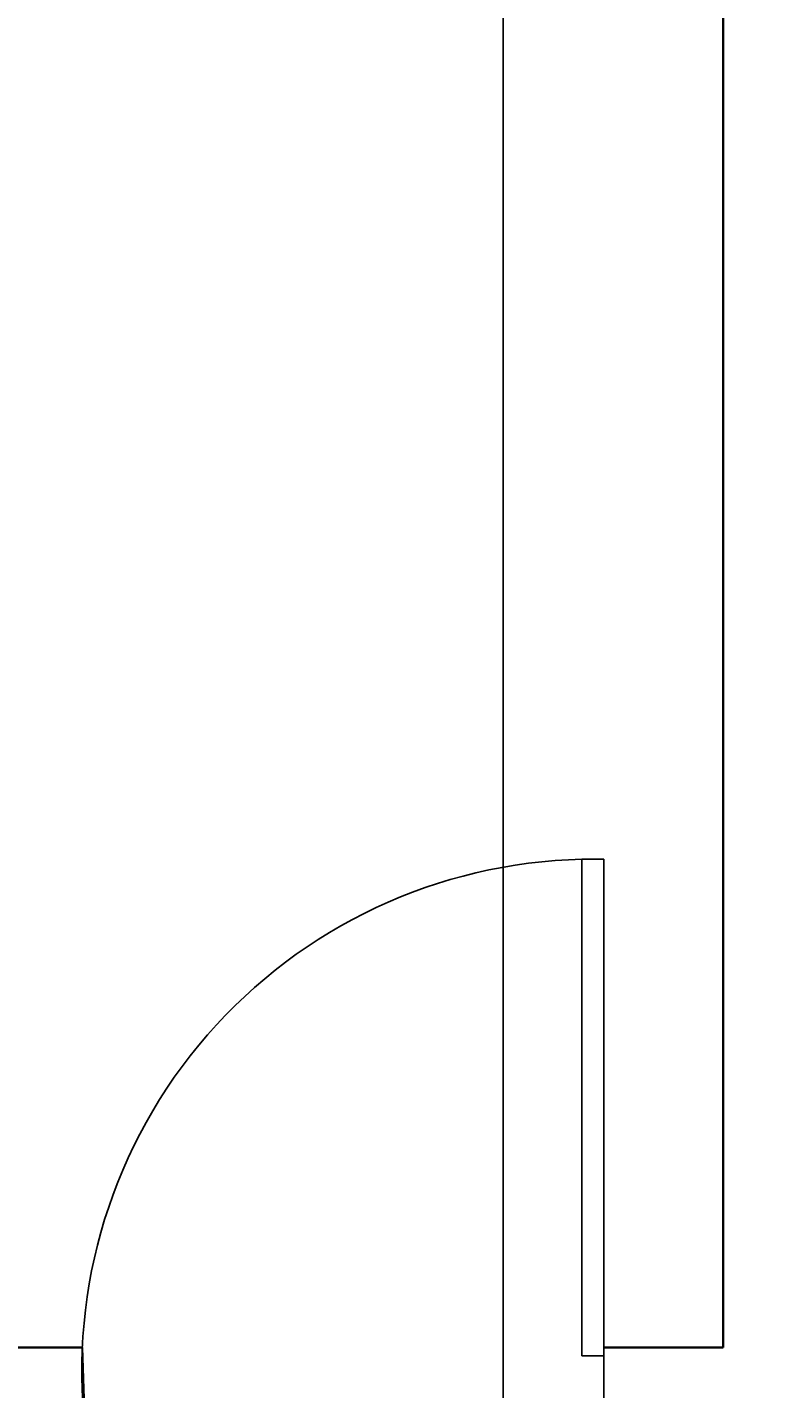
# Model space of a CAD drawing. Units: inches. Extents: x -61 to 1599, y -1316 to 257.
# Tile 122 of 204: x 181 to 236, y -10 to 88. Entities that reach past the tile are written whole.
import ezdxf

# ---------------------------------------------------------------- set-up
doc = ezdxf.new("R2010")
doc.units = ezdxf.units.IN
doc.header["$MEASUREMENT"] = 0
doc.linetypes.add('ACAD_ISO02W100', pattern=[15, 12, -3])
for name, color, linetype, lineweight in [('A-ANNO-DIMS', 2, 'Continuous', 18), ('A-WALL-JAMB', 4, 'ACAD_ISO02W100', 25), ('DOORS', 2, 'Continuous', 25), ('WALLS', 4, 'Continuous', 35)]:
    doc.layers.add(name, color=color, linetype=linetype, lineweight=lineweight)
doc.styles.get("Standard").update_dxf_attribs({"font": 'arial.ttf'})
doc.dimstyles.get("Standard").update_dxf_attribs({"dimtxt": 0.18, "dimasz": 0.18, "dimexe": 0.18, "dimexo": 0.0625, "dimgap": 0.09, "dimtad": 0, "dimtih": 1, "dimtoh": 1, "dimdec": 0, "dimzin": 0, "dimdsep": 46, "dimlunit": 3, "dimtxsty": 'Standard', "dimcen": 0.09, "dimadec": 0, "dimazin": 0, "dimtfac": 1, "dimtdec": 0, "dimtofl": 0, "dimtmove": 0, "dimatfit": 3, "dimfxl": 1, "dimtolj": 1, "dimtzin": 0, "dimarcsym": 0})

# ---------------------------------------------------------------- blocks, each defined once
blk = doc.blocks.new('DOOR-SWING-36')
blk.add_line((0, 0), (0, -5.4))
blk.add_lwpolyline([(0, 0), (0, 36), (-1.575, 36), (-1.575, 0)], close=True)
blk.add_arc((-0.739, -1.079), 37.088, 91.2913, 186.69053)
blk = doc.blocks.new('*D687')
at = {"layer": 'A-ANNO-DIMS', "color": 0, "lineweight": -2, "transparency": 16777216}
for p, q in [((289.418, 181.677), (-61.077, 181.677)), ((-60.897, 181.497), (-60.897, -528.952)), ((-60.897, -1239.765), (-60.897, -529.316)), ((319.64, -1239.945), (-61.077, -1239.945))]:
    blk.add_line(p, q, dxfattribs=at)
at = {"layer": 'A-ANNO-DIMS', "color": 0, "transparency": 16777216}
for points in [[(-60.927, 181.497), (-60.867, 181.497), (-60.897, 181.677)], [(-60.927, -1239.765), (-60.867, -1239.765), (-60.897, -1239.945)]]:
    blk.add_solid(points, dxfattribs=at)
at = {"layer": 'DEFPOINTS', "color": 0, "transparency": 16777216}
for p in [(289.481, 181.677), (-60.897, -1239.945), (319.703, -1239.945)]:
    blk.add_point(p, dxfattribs=at)
at = {"layer": 'A-ANNO-DIMS', "color": 0, "transparency": 16777216, "insert": (-60.897, -529.134), "char_height": 0.18, "attachment_point": 5}
blk.add_mtext('\\A1;1421.6', dxfattribs=at)
blk = doc.blocks.new('*D701')
at = {"layer": 'A-ANNO-DIMS', "color": 0, "lineweight": -2, "transparency": 16777216}
for p, q in [((215.752, -616.882), (215.752, 257.457)), ((215.932, 257.277), (233.924, 257.277)), ((252.702, 257.277), (234.711, 257.277)), ((252.882, -616.882), (252.882, 257.457))]:
    blk.add_line(p, q, dxfattribs=at)
at = {"layer": 'A-ANNO-DIMS', "color": 0, "transparency": 16777216}
for points in [[(215.932, 257.307), (215.932, 257.247), (215.752, 257.277)], [(252.702, 257.307), (252.702, 257.247), (252.882, 257.277)]]:
    blk.add_solid(points, dxfattribs=at)
at = {"layer": 'DEFPOINTS', "color": 0, "transparency": 16777216}
for p in [(252.882, 257.277), (215.752, -616.945), (252.882, -616.945)]:
    blk.add_point(p, dxfattribs=at)
at = {"layer": 'A-ANNO-DIMS', "color": 0, "transparency": 16777216, "insert": (234.317, 257.277), "char_height": 0.18, "attachment_point": 5}
blk.add_mtext('\\A1;37.13', dxfattribs=at)

msp = doc.modelspace()

# ---------------------------------------------------------------- linework, layer by layer
at = {"layer": 'A-WALL-JAMB'}
for p, q in [((185.4756, -13.3229), (185.2611, -7.3229)), ((223.0506, -13.3229), (223.0506, -7.3229))]:
    msp.add_line(p, q, dxfattribs=at)
at = {"layer": 'WALLS'}
for p, q in [((231.7028, 148.6771), (231.7028, -7.3229)), ((87.7028, -7.3229), (185.2611, -7.3229)), ((223.0506, -7.3229), (231.7028, -7.3229))]:
    msp.add_line(p, q, dxfattribs=at)

# ---------------------------------------------------------------- block references
at = {"layer": 'DOORS'}
msp.add_blockref('DOOR-SWING-36', (223.0506, -7.9229), dxfattribs=at)

# ---------------------------------------------------------------- dimensions: what is measured, and where the dimension line sits
at = {"layer": 'A-ANNO-DIMS'}
dim = msp.add_linear_dim(base=(252.8825, 257.2771), p1=(215.7521, -616.9446), p2=(252.8825, -616.9446), dimstyle='Standard', override={"dimdec": 2, "dimlfac": 1, "dimrnd": 0, "dimzin": 0, "dimdsep": 46, "dimlunit": 2}, dxfattribs=at)
dim.commit()
dim.dimension.update_dxf_attribs({"geometry": '*D701', "text_midpoint": (234.3173, 257.2771)})
dim = msp.add_linear_dim(base=(-60.8972, -1239.9446), p1=(289.4807, 181.6771), p2=(319.7028, -1239.9446), angle=90, dimstyle='Standard', override={"dimdec": 1, "dimlfac": 1, "dimrnd": 0, "dimzin": 0, "dimdsep": 46, "dimlunit": 2}, dxfattribs=at)
dim.commit()
dim.dimension.update_dxf_attribs({"geometry": '*D687', "text_midpoint": (-60.8972, -529.1337)})

doc.saveas('drawing.dxf')
